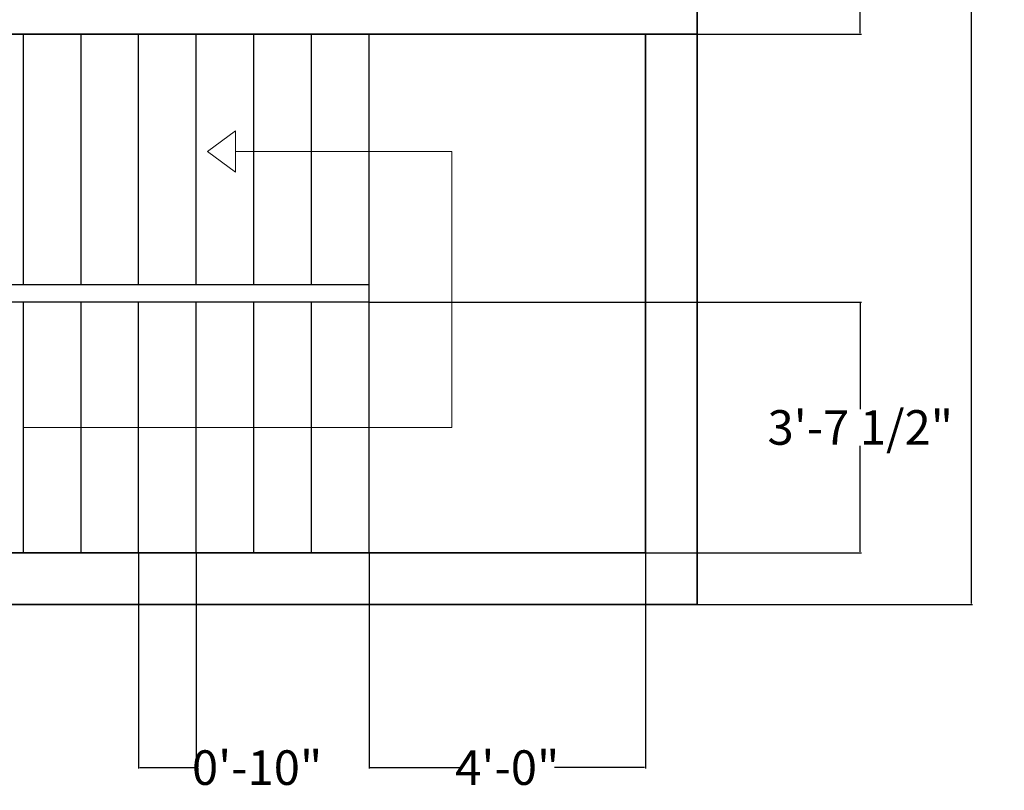
# Model space of a CAD drawing. Units: inches. Extents: x -26 to 575, y -18 to 513.
# Tile 16 of 28: x 405 to 575, y -13 to 121. Entities that reach past the tile are written whole.
import ezdxf

# ---------------------------------------------------------------- set-up
doc = ezdxf.new("R2010")
doc.units = ezdxf.units.IN
doc.header["$MEASUREMENT"] = 0
for name, color, linetype, lineweight in [('A-ANNO-DIMS', 2, 'Continuous', 18), ('A-ANNO-SYMB', 2, 'Continuous', 18), ('A-FLOR-STRS', 7, 'Continuous', 25), ('A-WALL', 7, 'Continuous', 35)]:
    doc.layers.add(name, color=color, linetype=linetype, lineweight=lineweight)
doc.styles.get("Standard").update_dxf_attribs({"font": 'arial.ttf', "height": 6})
doc.dimstyles.get("Standard").update_dxf_attribs({"dimtxt": 6, "dimasz": 0.18, "dimexe": 0.18, "dimexo": 0.0625, "dimgap": 0.09, "dimtad": 0, "dimtih": 1, "dimtoh": 1, "dimzin": 0, "dimdsep": 46, "dimlunit": 3, "dimtxsty": 'Standard', "dimcen": 0.09, "dimadec": 0, "dimazin": 0, "dimtfac": 1, "dimtofl": 0, "dimtmove": 0, "dimatfit": 3, "dimfxl": 1, "dimtolj": 1, "dimtzin": 0, "dimarcsym": 0})

# ---------------------------------------------------------------- blocks, each defined once
blk = doc.blocks.new('*D2')
at = {"layer": 'A-ANNO-DIMS', "color": 0, "lineweight": -2, "transparency": 16777216}
for p, q in [((522.24, 475.51), (569.98, 475.51)), ((569.8, 475.33), (569.8, 250.66)), ((569.8, 19.69), (569.8, 244.35)), ((522.24, 19.51), (569.98, 19.51))]:
    blk.add_line(p, q, dxfattribs=at)
at = {"layer": 'A-ANNO-DIMS', "color": 0, "transparency": 16777216}
for points in [[(569.77, 475.33), (569.83, 475.33), (569.8, 475.51)], [(569.77, 19.69), (569.83, 19.69), (569.8, 19.51)]]:
    blk.add_solid(points, dxfattribs=at)
at = {"layer": 'Defpoints', "color": 0, "transparency": 16777216}
for p in [(522.18, 475.51), (522.18, 19.51), (569.8, 19.51)]:
    blk.add_point(p, dxfattribs=at)
at = {"layer": 'A-ANNO-DIMS', "color": 0, "transparency": 16777216, "insert": (569.8, 247.51), "char_height": 6, "attachment_point": 5}
blk.add_mtext("\\A1;38'", dxfattribs=at)
blk = doc.blocks.new('*D35')
at = {"layer": 'A-ANNO-DIMS', "color": 0, "lineweight": -2, "transparency": 16777216}
for p, q in [((465.24, 72.01), (550.66, 72.01)), ((550.48, 71.83), (550.48, 53.45)), ((550.48, 28.69), (550.48, 47.06)), ((465.24, 28.51), (550.66, 28.51))]:
    blk.add_line(p, q, dxfattribs=at)
at = {"layer": 'A-ANNO-DIMS', "color": 0, "transparency": 16777216}
for points in [[(550.45, 71.83), (550.51, 71.83), (550.48, 72.01)], [(550.45, 28.69), (550.51, 28.69), (550.48, 28.51)]]:
    blk.add_solid(points, dxfattribs=at)
at = {"layer": 'Defpoints', "color": 0, "transparency": 16777216}
for p in [(465.18, 72.01), (550.48, 72.01), (465.18, 28.51)]:
    blk.add_point(p, dxfattribs=at)
at = {"layer": 'A-ANNO-DIMS', "color": 0, "transparency": 16777216, "insert": (550.48, 50.26), "char_height": 6, "attachment_point": 5}
blk.add_mtext('\\A1;3\'-7 1/2"', dxfattribs=at)
blk = doc.blocks.new('*D42')
at = {"layer": 'A-ANNO-DIMS', "color": 0, "lineweight": -2, "transparency": 16777216}
for p, q in [((522.24, 156.93), (550.66, 156.93)), ((550.48, 156.75), (550.48, 140.92)), ((550.48, 118.69), (550.48, 134.53)), ((522.24, 118.51), (550.66, 118.51))]:
    blk.add_line(p, q, dxfattribs=at)
at = {"layer": 'A-ANNO-DIMS', "color": 0, "transparency": 16777216}
for points in [[(550.45, 156.75), (550.51, 156.75), (550.48, 156.93)], [(550.45, 118.69), (550.51, 118.69), (550.48, 118.51)]]:
    blk.add_solid(points, dxfattribs=at)
at = {"layer": 'Defpoints', "color": 0, "transparency": 16777216}
for p in [(522.18, 156.93), (522.18, 118.51), (550.48, 118.51)]:
    blk.add_point(p, dxfattribs=at)
at = {"layer": 'A-ANNO-DIMS', "color": 0, "transparency": 16777216, "insert": (550.48, 137.72), "char_height": 6, "attachment_point": 5}
blk.add_mtext('\\A1;3\'-2 1/2"', dxfattribs=at)
blk = doc.blocks.new('*D44')
at = {"layer": 'A-ANNO-DIMS', "color": 0, "lineweight": -2, "transparency": 16777216}
for p, q in [((465.18, 28.45), (465.18, -8.97)), ((513.18, 28.45), (513.18, -8.97)), ((465.36, -8.79), (480.99, -8.79)), ((513, -8.79), (497.36, -8.79))]:
    blk.add_line(p, q, dxfattribs=at)
at = {"layer": 'A-ANNO-DIMS', "color": 0, "transparency": 16777216}
for points in [[(465.36, -8.76), (465.36, -8.82), (465.18, -8.79)], [(513, -8.76), (513, -8.82), (513.18, -8.79)]]:
    blk.add_solid(points, dxfattribs=at)
at = {"layer": 'Defpoints', "color": 0, "transparency": 16777216}
for p in [(465.18, 28.51), (513.18, 28.51), (513.18, -8.79)]:
    blk.add_point(p, dxfattribs=at)
at = {"layer": 'A-ANNO-DIMS', "color": 0, "transparency": 16777216, "insert": (489.18, -8.79), "char_height": 6, "attachment_point": 5}
blk.add_mtext('\\A1;4\'-0"', dxfattribs=at)
blk = doc.blocks.new('*D45')
at = {"layer": 'A-ANNO-DIMS', "color": 0, "lineweight": -2, "transparency": 16777216}
for p, q in [((425.18, 28.45), (425.18, -8.97)), ((435.18, 28.45), (435.18, -8.97)), ((425.36, -8.79), (435, -8.79)), ((435.18, -8.79), (435.36, -8.79))]:
    blk.add_line(p, q, dxfattribs=at)
at = {"layer": 'A-ANNO-DIMS', "color": 0, "transparency": 16777216}
for points in [[(425.36, -8.76), (425.36, -8.82), (425.18, -8.79)], [(435, -8.76), (435, -8.82), (435.18, -8.79)]]:
    blk.add_solid(points, dxfattribs=at)
at = {"layer": 'Defpoints', "color": 0, "transparency": 16777216}
for p in [(425.18, 28.51), (435.18, 28.51), (435.18, -8.79)]:
    blk.add_point(p, dxfattribs=at)
at = {"layer": 'A-ANNO-DIMS', "color": 0, "transparency": 16777216, "insert": (445.75, -8.79), "char_height": 6, "attachment_point": 5}
blk.add_mtext('\\A1;0\'-10"', dxfattribs=at)

msp = doc.modelspace()

# ---------------------------------------------------------------- linework, layer by layer
at = {"layer": 'A-ANNO-SYMB'}
for p, q in [((441.98, 101.735), (437.122, 98.169)), ((441.98, 98.169), (441.98, 101.735)), ((441.98, 94.603), (437.122, 98.169)), ((479.571, 98.169), (441.98, 98.169)), ((441.98, 98.169), (441.98, 94.603)), ((479.571, 50.258), (479.571, 98.169)), ((405.177, 50.258), (479.571, 50.258))]:
    msp.add_line(p, q, dxfattribs=at)
at = {"layer": 'A-FLOR-STRS'}
for p, q in [((405.177, 75.008), (405.177, 118.508)), ((415.177, 75.008), (415.177, 118.508)), ((425.177, 75.008), (425.177, 118.508)), ((435.177, 75.008), (435.177, 118.508)), ((445.177, 75.008), (445.177, 118.508)), ((455.177, 75.008), (455.177, 118.508)), ((465.177, 28.508), (465.177, 118.508)), ((465.177, 75.008), (365.177, 75.008)), ((465.177, 72.008), (365.177, 72.008)), ((405.177, 28.508), (405.177, 72.008)), ((415.177, 28.508), (415.177, 72.008)), ((425.177, 28.508), (425.177, 72.008)), ((435.177, 28.508), (435.177, 72.008)), ((445.177, 28.508), (445.177, 72.008)), ((455.177, 28.508), (455.177, 72.008))]:
    msp.add_line(p, q, dxfattribs=at)
at = {"layer": 'A-WALL'}
for p, q in [((522.177, 118.508), (360.409, 118.508)), ((513.177, 28.508), (513.177, 118.508)), ((27.177, 28.508), (513.177, 28.508))]:
    msp.add_line(p, q, dxfattribs=at)
msp.add_lwpolyline([(18.177, 19.508), (522.177, 19.508), (522.177, 475.508), (18.177, 475.508)], close=True, dxfattribs=at)

# ---------------------------------------------------------------- dimensions: what is measured, and where the dimension line sits
at = {"layer": 'A-ANNO-DIMS'}
for base, p1, p2, override, picture, middle in [((569.801, 19.508), (522.177, 475.508), (522.177, 19.508), {"dimclrd": 0, "dimclre": 0, "dimclrt": 0}, '*D2', (569.801, 247.508)), ((550.477, 118.508), (522.177, 156.934), (522.177, 118.508), {"dimdec": 1, "dimlfac": 1, "dimrnd": 0, "dimzin": 1, "dimdsep": 46, "dimlunit": 4, "dimfrac": 2}, '*D42', (550.477, 137.721)), ((550.477, 72.008), (465.177, 28.508), (465.177, 72.008), {"dimdec": 1, "dimlfac": 1, "dimrnd": 0, "dimzin": 1, "dimdsep": 46, "dimlunit": 4, "dimfrac": 2}, '*D35', (550.477, 50.258))]:
    dim = msp.add_linear_dim(base=base, p1=p1, p2=p2, angle=90, dimstyle='Standard', override=override, dxfattribs=at)
    dim.commit()
    dim.dimension.update_dxf_attribs({"geometry": picture, "text_midpoint": middle})
for base, p1, p2, picture, middle in [((435.177, -8.792), (425.177, 28.508), (435.177, 28.508), '*D45', (445.753, -8.792)), ((513.177, -8.792), (465.177, 28.508), (513.177, 28.508), '*D44', (489.177, -8.792))]:
    dim = msp.add_linear_dim(base=base, p1=p1, p2=p2, dimstyle='Standard', override={"dimdec": 1, "dimlfac": 1, "dimrnd": 0, "dimzin": 1, "dimdsep": 46, "dimlunit": 4, "dimfrac": 2}, dxfattribs=at)
    dim.commit()
    dim.dimension.update_dxf_attribs({"geometry": picture, "text_midpoint": middle})

doc.saveas('drawing.dxf')
